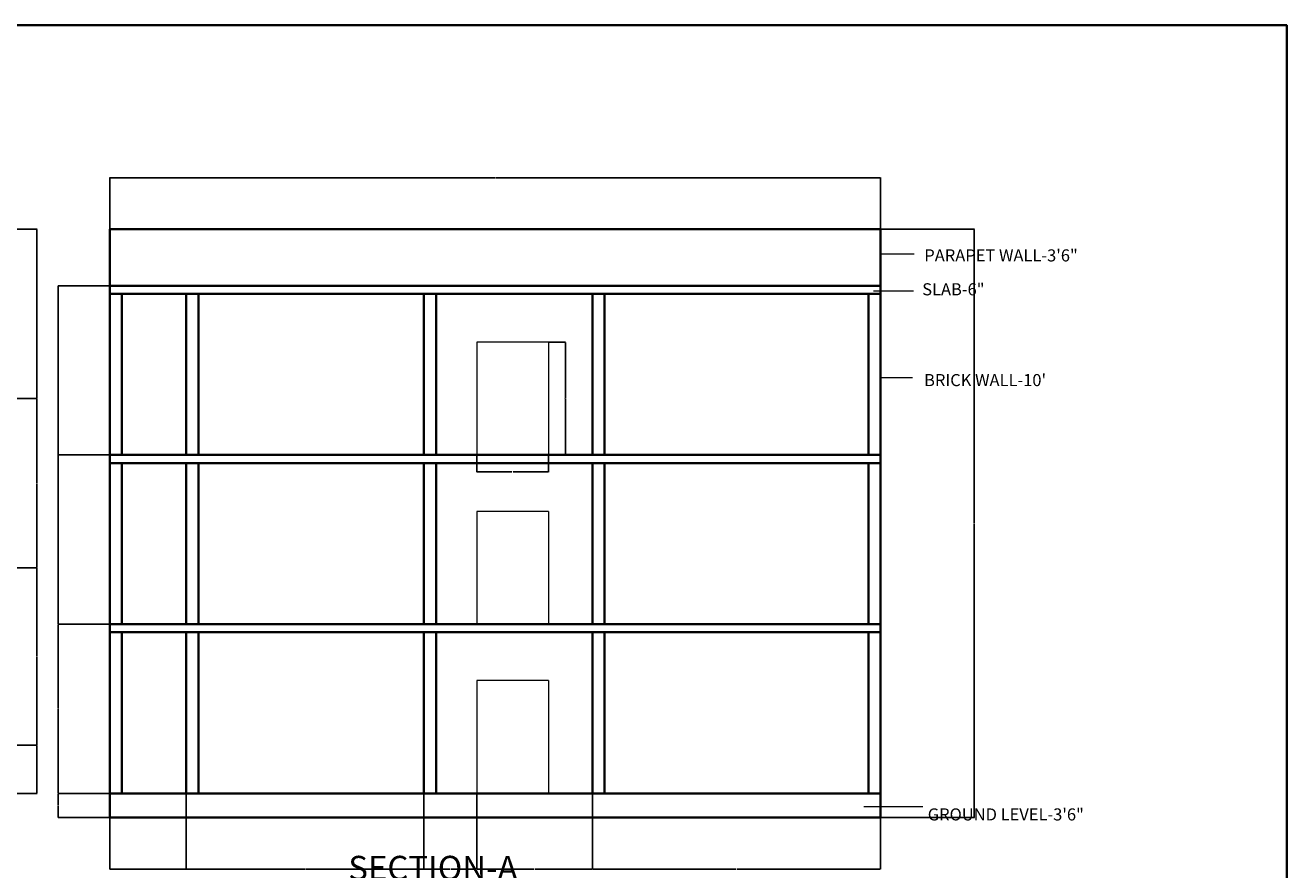
# Model space of a CAD drawing. Units: inches. Extents: x 1824 to 3509, y 619 to 2294.
# Tile 12 of 12: x 2570 to 3509, y 1665 to 2294. Entities that reach past the tile are written whole.
import ezdxf

# ---------------------------------------------------------------- set-up
doc = ezdxf.new("R2010")
doc.units = ezdxf.units.IN
for name, color, linetype, lineweight in [('A-ANNO-DIMS', 2, 'Continuous', 18), ('A-ANNO-SYMB', 7, 'Continuous', 18), ('A-ANNO-TEXT', 7, 'Continuous', 25), ('A-ANNO-TTLB', 7, 'Continuous', 35), ('A-SECT', 7, 'Continuous', 35), ('A-SECT-DOOR', 3, 'Continuous', 18)]:
    doc.layers.add(name, color=color, linetype=linetype, lineweight=lineweight)
doc.styles.get("Standard").update_dxf_attribs({"font": 'arial.ttf'})
doc.dimstyles.get("Standard").update_dxf_attribs({"dimtxt": 0.18, "dimasz": 0.18, "dimexe": 0.18, "dimexo": 0.0625, "dimgap": 0.09, "dimtad": 0, "dimtih": 1, "dimtoh": 1, "dimdec": 4, "dimzin": 0, "dimdsep": 46, "dimtxsty": 'Standard', "dimcen": 0.09, "dimadec": 0, "dimazin": 0, "dimtfac": 1, "dimtdec": 4, "dimtofl": 0, "dimtmove": 0, "dimatfit": 3, "dimfxl": 1, "dimtolj": 1, "dimtzin": 0, "dimarcsym": 0})

# ---------------------------------------------------------------- blocks, each defined once
blk = doc.blocks.new('DOOR-OPENING-SECT')
for p, q in [((0, 84), (0, 0)), ((53.41, 84), (0, 84)), ((53.41, 84), (53.41, 0))]:
    blk.add_line(p, q)
blk = doc.blocks.new('*D48')
at = {"layer": 'A-ANNO-DIMS', "color": 0, "lineweight": -2, "transparency": 16777216}
for p, q in [((2959.55, 2057.75), (2972.27, 2057.75)), ((2972.09, 2057.57), (2972.09, 2015.94)), ((2972.09, 1973.93), (2972.09, 2015.57)), ((2959.55, 1973.75), (2972.27, 1973.75))]:
    blk.add_line(p, q, dxfattribs=at)
at = {"layer": 'A-ANNO-DIMS', "color": 0, "transparency": 16777216}
for points in [[(2972.06, 2057.57), (2972.12, 2057.57), (2972.09, 2057.75)], [(2972.06, 1973.93), (2972.12, 1973.93), (2972.09, 1973.75)]]:
    blk.add_solid(points, dxfattribs=at)
at = {"layer": 'Defpoints', "color": 0, "transparency": 16777216}
for p in [(2959.49, 2057.75), (2972.09, 2057.75), (2959.49, 1973.75)]:
    blk.add_point(p, dxfattribs=at)
at = {"layer": 'A-ANNO-DIMS', "color": 0, "transparency": 16777216, "insert": (2972.09, 2015.75), "char_height": 0.18, "attachment_point": 5}
blk.add_mtext('\\A1;OPENING 84 TYP.', dxfattribs=at)
blk = doc.blocks.new('*D49')
at = {"layer": 'A-ANNO-DIMS', "color": 0, "lineweight": -2, "transparency": 16777216}
for p, q in [((2906.08, 1973.69), (2906.08, 1960.97)), ((2959.49, 1973.69), (2959.49, 1960.97)), ((2906.26, 1961.15), (2932.25, 1961.15)), ((2959.31, 1961.15), (2933.31, 1961.15))]:
    blk.add_line(p, q, dxfattribs=at)
at = {"layer": 'A-ANNO-DIMS', "color": 0, "transparency": 16777216}
for points in [[(2906.26, 1961.18), (2906.26, 1961.12), (2906.08, 1961.15)], [(2959.31, 1961.18), (2959.31, 1961.12), (2959.49, 1961.15)]]:
    blk.add_solid(points, dxfattribs=at)
at = {"layer": 'Defpoints', "color": 0, "transparency": 16777216}
for p in [(2906.08, 1973.75), (2959.49, 1973.75), (2959.49, 1961.15)]:
    blk.add_point(p, dxfattribs=at)
at = {"layer": 'A-ANNO-DIMS', "color": 0, "transparency": 16777216, "insert": (2932.78, 1961.15), "char_height": 0.18, "attachment_point": 5}
blk.add_mtext('\\A1;53 TYP.', dxfattribs=at)
blk = doc.blocks.new('*D126')
at = {"layer": 'A-ANNO-DIMS', "color": 0, "lineweight": -2, "transparency": 16777216}
for p, q in [((2447.72, 1757.75), (2578.67, 1757.75)), ((2578.49, 1757.57), (2578.49, 1739.93)), ((2578.49, 1721.93), (2578.49, 1739.57)), ((2523.15, 1721.75), (2578.67, 1721.75))]:
    blk.add_line(p, q, dxfattribs=at)
at = {"layer": 'A-ANNO-DIMS', "color": 0, "transparency": 16777216}
for points in [[(2578.46, 1757.57), (2578.52, 1757.57), (2578.49, 1757.75)], [(2578.46, 1721.93), (2578.52, 1721.93), (2578.49, 1721.75)]]:
    blk.add_solid(points, dxfattribs=at)
at = {"layer": 'Defpoints', "color": 0, "transparency": 16777216}
for p in [(2447.66, 1757.75), (2578.49, 1757.75), (2523.09, 1721.75)]:
    blk.add_point(p, dxfattribs=at)
at = {"layer": 'A-ANNO-DIMS', "color": 0, "transparency": 16777216, "insert": (2578.49, 1739.75), "char_height": 0.18, "attachment_point": 5}
blk.add_mtext('\\A1;36', dxfattribs=at)
blk = doc.blocks.new('*D127')
at = {"layer": 'A-ANNO-DIMS', "color": 0, "lineweight": -2, "transparency": 16777216}
for p, q in [((2547.15, 1889.75), (2578.67, 1889.75)), ((2578.49, 1889.57), (2578.49, 1823.93)), ((2578.49, 1757.93), (2578.49, 1823.57)), ((2447.72, 1757.75), (2578.67, 1757.75))]:
    blk.add_line(p, q, dxfattribs=at)
at = {"layer": 'A-ANNO-DIMS', "color": 0, "transparency": 16777216}
for points in [[(2578.46, 1889.57), (2578.52, 1889.57), (2578.49, 1889.75)], [(2578.46, 1757.93), (2578.52, 1757.93), (2578.49, 1757.75)]]:
    blk.add_solid(points, dxfattribs=at)
at = {"layer": 'Defpoints', "color": 0, "transparency": 16777216}
for p in [(2547.09, 1889.75), (2578.49, 1889.75), (2447.66, 1757.75)]:
    blk.add_point(p, dxfattribs=at)
at = {"layer": 'A-ANNO-DIMS', "color": 0, "transparency": 16777216, "insert": (2578.49, 1823.75), "char_height": 0.18, "attachment_point": 5}
blk.add_mtext('\\A1;132', dxfattribs=at)
blk = doc.blocks.new('*D128')
at = {"layer": 'A-ANNO-DIMS', "color": 0, "lineweight": -2, "transparency": 16777216}
for p, q in [((2547.15, 2015.75), (2578.67, 2015.75)), ((2578.49, 2015.57), (2578.49, 1952.93)), ((2578.49, 1889.93), (2578.49, 1952.57)), ((2547.15, 1889.75), (2578.67, 1889.75))]:
    blk.add_line(p, q, dxfattribs=at)
at = {"layer": 'A-ANNO-DIMS', "color": 0, "transparency": 16777216}
for points in [[(2578.46, 2015.57), (2578.52, 2015.57), (2578.49, 2015.75)], [(2578.46, 1889.93), (2578.52, 1889.93), (2578.49, 1889.75)]]:
    blk.add_solid(points, dxfattribs=at)
at = {"layer": 'Defpoints', "color": 0, "transparency": 16777216}
for p in [(2547.09, 2015.75), (2578.49, 2015.75), (2547.09, 1889.75)]:
    blk.add_point(p, dxfattribs=at)
at = {"layer": 'A-ANNO-DIMS', "color": 0, "transparency": 16777216, "insert": (2578.49, 1952.75), "char_height": 0.18, "attachment_point": 5}
blk.add_mtext('\\A1;126', dxfattribs=at)
blk = doc.blocks.new('*D129')
at = {"layer": 'A-ANNO-DIMS', "color": 0, "lineweight": -2, "transparency": 16777216}
for p, q in [((2547.15, 2141.75), (2578.67, 2141.75)), ((2578.49, 2141.57), (2578.49, 2078.93)), ((2578.49, 2015.93), (2578.49, 2078.57)), ((2547.15, 2015.75), (2578.67, 2015.75))]:
    blk.add_line(p, q, dxfattribs=at)
at = {"layer": 'A-ANNO-DIMS', "color": 0, "transparency": 16777216}
for points in [[(2578.46, 2141.57), (2578.52, 2141.57), (2578.49, 2141.75)], [(2578.46, 2015.93), (2578.52, 2015.93), (2578.49, 2015.75)]]:
    blk.add_solid(points, dxfattribs=at)
at = {"layer": 'Defpoints', "color": 0, "transparency": 16777216}
for p in [(2547.09, 2141.75), (2578.49, 2141.75), (2547.09, 2015.75)]:
    blk.add_point(p, dxfattribs=at)
at = {"layer": 'A-ANNO-DIMS', "color": 0, "transparency": 16777216, "insert": (2578.49, 2078.75), "char_height": 0.18, "attachment_point": 5}
blk.add_mtext('\\A1;126', dxfattribs=at)
blk = doc.blocks.new('*D130')
at = {"layer": 'A-ANNO-DIMS', "color": 0, "lineweight": -2, "transparency": 16777216}
for p, q in [((2632.73, 2141.81), (2632.73, 2180.23)), ((2632.91, 2180.05), (2919.44, 2180.05)), ((3206.55, 2180.05), (2920.02, 2180.05)), ((3206.73, 2141.81), (3206.73, 2180.23))]:
    blk.add_line(p, q, dxfattribs=at)
at = {"layer": 'A-ANNO-DIMS', "color": 0, "transparency": 16777216}
for points in [[(2632.91, 2180.08), (2632.91, 2180.02), (2632.73, 2180.05)], [(3206.55, 2180.08), (3206.55, 2180.02), (3206.73, 2180.05)]]:
    blk.add_solid(points, dxfattribs=at)
at = {"layer": 'Defpoints', "color": 0, "transparency": 16777216}
for p in [(3206.73, 2180.05), (2632.73, 2141.75), (3206.73, 2141.75)]:
    blk.add_point(p, dxfattribs=at)
at = {"layer": 'A-ANNO-DIMS', "color": 0, "transparency": 16777216, "insert": (2919.73, 2180.05), "char_height": 0.18, "attachment_point": 5}
blk.add_mtext('\\A1;574', dxfattribs=at)
blk = doc.blocks.new('*D131')
at = {"layer": 'A-ANNO-DIMS', "color": 0, "lineweight": -2, "transparency": 16777216}
for p, q in [((3206.79, 2141.75), (3276.71, 2141.75)), ((3276.53, 2141.57), (3276.53, 1922.93)), ((3276.53, 1703.93), (3276.53, 1922.57)), ((3206.79, 1703.75), (3276.71, 1703.75))]:
    blk.add_line(p, q, dxfattribs=at)
at = {"layer": 'A-ANNO-DIMS', "color": 0, "transparency": 16777216}
for points in [[(3276.5, 2141.57), (3276.56, 2141.57), (3276.53, 2141.75)], [(3276.5, 1703.93), (3276.56, 1703.93), (3276.53, 1703.75)]]:
    blk.add_solid(points, dxfattribs=at)
at = {"layer": 'Defpoints', "color": 0, "transparency": 16777216}
for p in [(3206.73, 2141.75), (3276.53, 2141.75), (3206.73, 1703.75)]:
    blk.add_point(p, dxfattribs=at)
at = {"layer": 'A-ANNO-DIMS', "color": 0, "transparency": 16777216, "insert": (3276.53, 1922.75), "char_height": 0.18, "attachment_point": 5}
blk.add_mtext('\\A1;438', dxfattribs=at)
blk = doc.blocks.new('*D132')
at = {"layer": 'A-ANNO-DIMS', "color": 0, "lineweight": -2, "transparency": 16777216}
for p, q in [((2632.67, 1721.75), (2594.25, 1721.75)), ((2594.43, 1721.57), (2594.43, 1712.93)), ((2594.43, 1703.93), (2594.43, 1712.57)), ((2632.67, 1703.75), (2594.25, 1703.75))]:
    blk.add_line(p, q, dxfattribs=at)
at = {"layer": 'A-ANNO-DIMS', "color": 0, "transparency": 16777216}
for points in [[(2594.4, 1721.57), (2594.46, 1721.57), (2594.43, 1721.75)], [(2594.4, 1703.93), (2594.46, 1703.93), (2594.43, 1703.75)]]:
    blk.add_solid(points, dxfattribs=at)
at = {"layer": 'Defpoints', "color": 0, "transparency": 16777216}
for p in [(2594.43, 1721.75), (2632.73, 1721.75), (2632.73, 1703.75)]:
    blk.add_point(p, dxfattribs=at)
at = {"layer": 'A-ANNO-DIMS', "color": 0, "transparency": 16777216, "insert": (2594.43, 1712.75), "char_height": 0.18, "attachment_point": 5}
blk.add_mtext('\\A1;18', dxfattribs=at)
blk = doc.blocks.new('*D133')
at = {"layer": 'A-ANNO-DIMS', "color": 0, "lineweight": -2, "transparency": 16777216}
for p, q in [((2632.67, 1847.75), (2594.25, 1847.75)), ((2594.43, 1847.57), (2594.43, 1784.93)), ((2594.43, 1721.93), (2594.43, 1784.57)), ((2632.67, 1721.75), (2594.25, 1721.75))]:
    blk.add_line(p, q, dxfattribs=at)
at = {"layer": 'A-ANNO-DIMS', "color": 0, "transparency": 16777216}
for points in [[(2594.4, 1847.57), (2594.46, 1847.57), (2594.43, 1847.75)], [(2594.4, 1721.93), (2594.46, 1721.93), (2594.43, 1721.75)]]:
    blk.add_solid(points, dxfattribs=at)
at = {"layer": 'Defpoints', "color": 0, "transparency": 16777216}
for p in [(2594.43, 1847.75), (2632.73, 1847.75), (2632.73, 1721.75)]:
    blk.add_point(p, dxfattribs=at)
at = {"layer": 'A-ANNO-DIMS', "color": 0, "transparency": 16777216, "insert": (2594.43, 1784.75), "char_height": 0.18, "attachment_point": 5}
blk.add_mtext('\\A1;126', dxfattribs=at)
blk = doc.blocks.new('*D134')
at = {"layer": 'A-ANNO-DIMS', "color": 0, "lineweight": -2, "transparency": 16777216}
for p, q in [((2632.67, 1973.75), (2594.25, 1973.75)), ((2594.43, 1973.57), (2594.43, 1910.93)), ((2594.43, 1847.93), (2594.43, 1910.57)), ((2632.67, 1847.75), (2594.25, 1847.75))]:
    blk.add_line(p, q, dxfattribs=at)
at = {"layer": 'A-ANNO-DIMS', "color": 0, "transparency": 16777216}
for points in [[(2594.4, 1973.57), (2594.46, 1973.57), (2594.43, 1973.75)], [(2594.4, 1847.93), (2594.46, 1847.93), (2594.43, 1847.75)]]:
    blk.add_solid(points, dxfattribs=at)
at = {"layer": 'Defpoints', "color": 0, "transparency": 16777216}
for p in [(2594.43, 1973.75), (2632.73, 1973.75), (2632.73, 1847.75)]:
    blk.add_point(p, dxfattribs=at)
at = {"layer": 'A-ANNO-DIMS', "color": 0, "transparency": 16777216, "insert": (2594.43, 1910.75), "char_height": 0.18, "attachment_point": 5}
blk.add_mtext('\\A1;126', dxfattribs=at)
blk = doc.blocks.new('*D135')
at = {"layer": 'A-ANNO-DIMS', "color": 0, "lineweight": -2, "transparency": 16777216}
for p, q in [((2632.67, 2099.75), (2594.25, 2099.75)), ((2594.43, 2099.57), (2594.43, 2036.93)), ((2594.43, 1973.93), (2594.43, 2036.57)), ((2632.67, 1973.75), (2594.25, 1973.75))]:
    blk.add_line(p, q, dxfattribs=at)
at = {"layer": 'A-ANNO-DIMS', "color": 0, "transparency": 16777216}
for points in [[(2594.4, 2099.57), (2594.46, 2099.57), (2594.43, 2099.75)], [(2594.4, 1973.93), (2594.46, 1973.93), (2594.43, 1973.75)]]:
    blk.add_solid(points, dxfattribs=at)
at = {"layer": 'Defpoints', "color": 0, "transparency": 16777216}
for p in [(2594.43, 2099.75), (2632.73, 2099.75), (2632.73, 1973.75)]:
    blk.add_point(p, dxfattribs=at)
at = {"layer": 'A-ANNO-DIMS', "color": 0, "transparency": 16777216, "insert": (2594.43, 2036.75), "char_height": 0.18, "attachment_point": 5}
blk.add_mtext('\\A1;126', dxfattribs=at)
blk = doc.blocks.new('*D136')
at = {"layer": 'A-ANNO-DIMS', "color": 0, "lineweight": -2, "transparency": 16777216}
for p, q in [((2689.73, 1721.69), (2689.73, 1665.27)), ((2632.73, 1703.69), (2632.73, 1665.27)), ((2632.91, 1665.45), (2661.01, 1665.45)), ((2689.55, 1665.45), (2661.45, 1665.45))]:
    blk.add_line(p, q, dxfattribs=at)
at = {"layer": 'A-ANNO-DIMS', "color": 0, "transparency": 16777216}
for points in [[(2632.91, 1665.48), (2632.91, 1665.42), (2632.73, 1665.45)], [(2689.55, 1665.48), (2689.55, 1665.42), (2689.73, 1665.45)]]:
    blk.add_solid(points, dxfattribs=at)
at = {"layer": 'Defpoints', "color": 0, "transparency": 16777216}
for p in [(2689.73, 1721.75), (2632.73, 1703.75), (2689.73, 1665.45)]:
    blk.add_point(p, dxfattribs=at)
at = {"layer": 'A-ANNO-DIMS', "color": 0, "transparency": 16777216, "insert": (2661.23, 1665.45), "char_height": 0.18, "attachment_point": 5}
blk.add_mtext('\\A1;57', dxfattribs=at)
blk = doc.blocks.new('*D137')
at = {"layer": 'A-ANNO-DIMS', "color": 0, "lineweight": -2, "transparency": 16777216}
for p, q in [((2689.73, 1721.69), (2689.73, 1665.27)), ((2866.73, 1721.69), (2866.73, 1665.27)), ((2689.91, 1665.45), (2777.95, 1665.45)), ((2866.55, 1665.45), (2778.51, 1665.45))]:
    blk.add_line(p, q, dxfattribs=at)
at = {"layer": 'A-ANNO-DIMS', "color": 0, "transparency": 16777216}
for points in [[(2689.91, 1665.48), (2689.91, 1665.42), (2689.73, 1665.45)], [(2866.55, 1665.48), (2866.55, 1665.42), (2866.73, 1665.45)]]:
    blk.add_solid(points, dxfattribs=at)
at = {"layer": 'Defpoints', "color": 0, "transparency": 16777216}
for p in [(2689.73, 1721.75), (2866.73, 1721.75), (2866.73, 1665.45)]:
    blk.add_point(p, dxfattribs=at)
at = {"layer": 'A-ANNO-DIMS', "color": 0, "transparency": 16777216, "insert": (2778.23, 1665.45), "char_height": 0.18, "attachment_point": 5}
blk.add_mtext('\\A1;177', dxfattribs=at)
blk = doc.blocks.new('*D138')
at = {"layer": 'A-ANNO-DIMS', "color": 0, "lineweight": -2, "transparency": 16777216}
for p, q in [((2866.73, 1721.69), (2866.73, 1665.27)), ((2906.08, 1721.69), (2906.08, 1665.27)), ((2866.91, 1665.45), (2886.01, 1665.45)), ((2905.9, 1665.45), (2886.8, 1665.45))]:
    blk.add_line(p, q, dxfattribs=at)
at = {"layer": 'A-ANNO-DIMS', "color": 0, "transparency": 16777216}
for points in [[(2866.91, 1665.48), (2866.91, 1665.42), (2866.73, 1665.45)], [(2905.9, 1665.48), (2905.9, 1665.42), (2906.08, 1665.45)]]:
    blk.add_solid(points, dxfattribs=at)
at = {"layer": 'Defpoints', "color": 0, "transparency": 16777216}
for p in [(2866.73, 1721.75), (2906.08, 1721.75), (2906.08, 1665.45)]:
    blk.add_point(p, dxfattribs=at)
at = {"layer": 'A-ANNO-DIMS', "color": 0, "transparency": 16777216, "insert": (2886.4, 1665.45), "char_height": 0.18, "attachment_point": 5}
blk.add_mtext('\\A1;39.35', dxfattribs=at)
blk = doc.blocks.new('*D139')
at = {"layer": 'A-ANNO-DIMS', "color": 0, "lineweight": -2, "transparency": 16777216}
for p, q in [((2906.08, 1721.69), (2906.08, 1665.27)), ((2992.23, 1721.69), (2992.23, 1665.27)), ((2906.26, 1665.45), (2948.76, 1665.45)), ((2992.05, 1665.45), (2949.55, 1665.45))]:
    blk.add_line(p, q, dxfattribs=at)
at = {"layer": 'A-ANNO-DIMS', "color": 0, "transparency": 16777216}
for points in [[(2906.26, 1665.48), (2906.26, 1665.42), (2906.08, 1665.45)], [(2992.05, 1665.48), (2992.05, 1665.42), (2992.23, 1665.45)]]:
    blk.add_solid(points, dxfattribs=at)
at = {"layer": 'Defpoints', "color": 0, "transparency": 16777216}
for p in [(2906.08, 1721.75), (2992.23, 1721.75), (2992.23, 1665.45)]:
    blk.add_point(p, dxfattribs=at)
at = {"layer": 'A-ANNO-DIMS', "color": 0, "transparency": 16777216, "insert": (2949.15, 1665.45), "char_height": 0.18, "attachment_point": 5}
blk.add_mtext('\\A1;86.15', dxfattribs=at)
blk = doc.blocks.new('*D140')
at = {"layer": 'A-ANNO-DIMS', "color": 0, "lineweight": -2, "transparency": 16777216}
for p, q in [((2992.23, 1721.69), (2992.23, 1665.27)), ((3206.73, 1703.69), (3206.73, 1665.27)), ((2992.41, 1665.45), (3099.08, 1665.45)), ((3206.55, 1665.45), (3099.87, 1665.45))]:
    blk.add_line(p, q, dxfattribs=at)
at = {"layer": 'A-ANNO-DIMS', "color": 0, "transparency": 16777216}
for points in [[(2992.41, 1665.48), (2992.41, 1665.42), (2992.23, 1665.45)], [(3206.55, 1665.48), (3206.55, 1665.42), (3206.73, 1665.45)]]:
    blk.add_solid(points, dxfattribs=at)
at = {"layer": 'Defpoints', "color": 0, "transparency": 16777216}
for p in [(2992.23, 1721.75), (3206.73, 1703.75), (3206.73, 1665.45)]:
    blk.add_point(p, dxfattribs=at)
at = {"layer": 'A-ANNO-DIMS', "color": 0, "transparency": 16777216, "insert": (3099.48, 1665.45), "char_height": 0.18, "attachment_point": 5}
blk.add_mtext('\\A1;214.5', dxfattribs=at)

msp = doc.modelspace()

# ---------------------------------------------------------------- linework, layer by layer
at = {"layer": 'A-ANNO-SYMB'}
for p, q in [((3206.7282, 2123.5094), (3231.9029, 2123.5094)), ((3201.6012, 2096.0059), (3231.4406, 2096.0059)), ((3206.7282, 2031.315), (3230.6619, 2031.315)), ((3194.4511, 1711.9835), (3238.2318, 1711.9835))]:
    msp.add_line(p, q, dxfattribs=at)
at = {"layer": 'A-ANNO-TTLB'}
msp.add_lwpolyline([(1824.0608, 2293.6614), (3509.3484, 2293.6614), (3509.3484, 619.4665), (1824.0608, 619.4665)], close=True, dxfattribs=at)
at = {"layer": 'A-SECT'}
for p, q in [((2632.7282, 2141.7521), (2632.7282, 1955.7521)), ((3206.7282, 2141.7521), (2632.7282, 2141.7521)), ((3206.7282, 2141.7521), (3206.7282, 1955.7521)), ((3206.7282, 2099.7521), (2632.7282, 2099.7521)), ((3206.7282, 2093.7521), (2632.7282, 2093.7521)), ((2641.7282, 2093.7521), (2641.7282, 1973.7521)), ((2689.7282, 2093.7521), (2689.7282, 1973.7521)), ((2689.7282, 2093.7521), (2689.7282, 1973.7521)), ((2698.7282, 2093.7521), (2698.7282, 1973.7521)), ((2698.7282, 2093.7521), (2698.7282, 1973.7521)), ((2866.7282, 2093.7521), (2866.7282, 1973.7521)), ((2875.7282, 2093.7521), (2875.7282, 1973.7521)), ((2992.2282, 2093.7521), (2992.2282, 1973.7521)), ((3001.2282, 2093.7521), (3001.2282, 1973.7521)), ((3197.7282, 2093.7521), (3197.7282, 1973.7521)), ((2632.7282, 2015.7521), (2632.7282, 1829.7521)), ((2632.7282, 2015.7521), (2632.7282, 1829.7521)), ((3206.7282, 2015.7521), (3206.7282, 1829.7521)), ((3206.7282, 2015.7521), (3206.7282, 1829.7521)), ((3206.7282, 1973.7521), (2632.7282, 1973.7521)), ((3206.7282, 1973.7521), (2632.7282, 1973.7521)), ((3206.7282, 1967.7521), (2632.7282, 1967.7521)), ((3206.7282, 1967.7521), (2632.7282, 1967.7521)), ((2641.7282, 1967.7521), (2641.7282, 1847.7521)), ((2641.7282, 1967.7521), (2641.7282, 1847.7521)), ((2689.7282, 1967.7521), (2689.7282, 1847.7521)), ((2689.7282, 1967.7521), (2689.7282, 1847.7521)), ((2689.7282, 1967.7521), (2689.7282, 1847.7521)), ((2689.7282, 1967.7521), (2689.7282, 1847.7521)), ((2698.7282, 1967.7521), (2698.7282, 1847.7521)), ((2698.7282, 1967.7521), (2698.7282, 1847.7521)), ((2698.7282, 1967.7521), (2698.7282, 1847.7521)), ((2698.7282, 1967.7521), (2698.7282, 1847.7521)), ((2866.7282, 1967.7521), (2866.7282, 1847.7521)), ((2866.7282, 1967.7521), (2866.7282, 1847.7521)), ((2875.7282, 1967.7521), (2875.7282, 1847.7521)), ((2875.7282, 1967.7521), (2875.7282, 1847.7521)), ((2992.2282, 1967.7521), (2992.2282, 1847.7521)), ((2992.2282, 1967.7521), (2992.2282, 1847.7521)), ((3001.2282, 1967.7521), (3001.2282, 1847.7521)), ((3001.2282, 1967.7521), (3001.2282, 1847.7521)), ((3197.7282, 1967.7521), (3197.7282, 1847.7521)), ((3197.7282, 1967.7521), (3197.7282, 1847.7521)), ((2632.7282, 1889.7521), (2632.7282, 1703.7521)), ((3206.7282, 1889.7521), (3206.7282, 1703.7521)), ((3206.7282, 1847.7521), (2632.7282, 1847.7521)), ((3206.7282, 1841.7521), (2632.7282, 1841.7521)), ((2641.7282, 1841.7521), (2641.7282, 1721.7521)), ((2689.7282, 1841.7521), (2689.7282, 1721.7521)), ((2689.7282, 1841.7521), (2689.7282, 1721.7521)), ((2698.7282, 1841.7521), (2698.7282, 1721.7521)), ((2698.7282, 1841.7521), (2698.7282, 1721.7521)), ((2866.7282, 1841.7521), (2866.7282, 1721.7521)), ((2875.7282, 1841.7521), (2875.7282, 1721.7521)), ((2992.2282, 1841.7521), (2992.2282, 1721.7521)), ((3001.2282, 1841.7521), (3001.2282, 1721.7521)), ((3197.7282, 1841.7521), (3197.7282, 1721.7521)), ((3206.7282, 1721.7521), (2632.7282, 1721.7521)), ((3206.7282, 1703.7521), (2632.7282, 1703.7521)), ((3206.7282, 1703.7521), (2632.7282, 1703.7521))]:
    msp.add_line(p, q, dxfattribs=at)

# ---------------------------------------------------------------- block references
at = {"layer": 'A-SECT-DOOR'}
for p in [(2906.078, 1973.752), (2906.078, 1847.752), (2906.078, 1847.752), (2906.078, 1721.752)]:
    msp.add_blockref('DOOR-OPENING-SECT', p, dxfattribs=at)

# ---------------------------------------------------------------- texts
at = {"layer": 'A-ANNO-TEXT', "attachment_point": 1}
for s, width, insert, char_height in [('PARAPET WALL-3\'6"', 341.336967, (3239.4028, 2126.8143), 9), ('SLAB-6"', 59.420797, (3237.8359, 2101.5868), 9), ("BRICK WALL-10'", 146.360884, (3239.2259, 2033.9854), 9), ('GROUND LEVEL-3\'6"', 171.746045, (3241.9663, 1710.647), 9), ('SECTION-A', 244.115567, (2810.3821, 1675.3119), 18)]:
    msp.add_mtext_dynamic_manual_height_columns(s, width=width, gutter_width=12.5, heights=[0], dxfattribs=dict(at, insert=insert, char_height=char_height))

# ---------------------------------------------------------------- dimensions: what is measured, and where the dimension line sits
at = {"layer": 'A-ANNO-DIMS'}
for base, p1, p2, override, picture, middle in [((3206.7282, 2180.0521), (2632.7282, 2141.7521), (3206.7282, 2141.7521), {"dimdec": 0, "dimlfac": 1, "dimrnd": 0, "dimzin": 0, "dimdsep": 46, "dimlunit": 2}, '*D130', (2919.7282, 2180.0521)), ((2689.7282, 1665.4521), (2632.7282, 1703.7521), (2689.7282, 1721.7521), {"dimdec": 0, "dimlfac": 1, "dimrnd": 0, "dimzin": 0, "dimdsep": 46, "dimlunit": 2}, '*D136', (2661.2282, 1665.4521)), ((2866.7282, 1665.4521), (2689.7282, 1721.7521), (2866.7282, 1721.7521), {"dimdec": 0, "dimlfac": 1, "dimrnd": 0, "dimzin": 0, "dimdsep": 46, "dimlunit": 2}, '*D137', (2778.2282, 1665.4521)), ((2906.0784, 1665.4521), (2866.7282, 1721.7521), (2906.0784, 1721.7521), {"dimdec": 2, "dimlfac": 1, "dimrnd": 0, "dimzin": 0, "dimdsep": 46, "dimlunit": 2}, '*D138', (2886.4033, 1665.4521)), ((2992.2282, 1665.4521), (2906.0784, 1721.7521), (2992.2282, 1721.7521), {"dimdec": 2, "dimlfac": 1, "dimrnd": 0, "dimzin": 0, "dimdsep": 46, "dimlunit": 2}, '*D139', (2949.1533, 1665.4521)), ((3206.7282, 1665.4521), (2992.2282, 1721.7521), (3206.7282, 1703.7521), {"dimdec": 1, "dimlfac": 1, "dimrnd": 0, "dimzin": 0, "dimdsep": 46, "dimlunit": 2}, '*D140', (3099.4782, 1665.4521))]:
    dim = msp.add_linear_dim(base=base, p1=p1, p2=p2, dimstyle='Standard', override=override, dxfattribs=at)
    dim.commit()
    dim.dimension.update_dxf_attribs({"geometry": picture, "text_midpoint": middle})
for base, p1, p2, picture, middle in [((2578.4899, 2141.7521), (2547.0899, 2015.7521), (2547.0899, 2141.7521), '*D129', (2578.4899, 2078.7521)), ((3276.5318, 2141.7521), (3206.7282, 1703.7521), (3206.7282, 2141.7521), '*D131', (3276.5318, 1922.7521)), ((2594.4282, 2099.7521), (2632.7282, 1973.7521), (2632.7282, 2099.7521), '*D135', (2594.4282, 2036.7521)), ((2578.4899, 2015.7521), (2547.0899, 1889.7521), (2547.0899, 2015.7521), '*D128', (2578.4899, 1952.7521)), ((2594.4282, 1973.7521), (2632.7282, 1847.7521), (2632.7282, 1973.7521), '*D134', (2594.4282, 1910.7521)), ((2578.4899, 1889.7521), (2447.6578, 1757.7521), (2547.0899, 1889.7521), '*D127', (2578.4899, 1823.7521)), ((2594.4282, 1847.7521), (2632.7282, 1721.7521), (2632.7282, 1847.7521), '*D133', (2594.4282, 1784.7521)), ((2578.4899, 1757.7521), (2523.0899, 1721.7521), (2447.6578, 1757.7521), '*D126', (2578.4899, 1739.7521)), ((2594.4282, 1721.7521), (2632.7282, 1703.7521), (2632.7282, 1721.7521), '*D132', (2594.4282, 1712.7521))]:
    dim = msp.add_linear_dim(base=base, p1=p1, p2=p2, angle=90, dimstyle='Standard', override={"dimdec": 0, "dimlfac": 1, "dimrnd": 0, "dimzin": 0, "dimdsep": 46, "dimlunit": 2}, dxfattribs=at)
    dim.commit()
    dim.dimension.update_dxf_attribs({"geometry": picture, "text_midpoint": middle})
dim = msp.add_linear_dim(base=(2972.0861, 2057.7521), p1=(2959.4861, 1973.7521), p2=(2959.4861, 2057.7521), angle=90, text='OPENING <> TYP.', dimstyle='Standard', override={"dimdec": 0, "dimlfac": 1, "dimrnd": 0, "dimzin": 0, "dimdsep": 46, "dimlunit": 2}, dxfattribs=at)
dim.commit()
dim.dimension.update_dxf_attribs({"geometry": '*D48', "text_midpoint": (2972.0861, 2015.7521)})
dim = msp.add_linear_dim(base=(2959.4861, 1961.1521), p1=(2906.0784, 1973.7521), p2=(2959.4861, 1973.7521), text='<> TYP.', dimstyle='Standard', override={"dimdec": 0, "dimlfac": 1, "dimrnd": 0, "dimzin": 0, "dimdsep": 46, "dimlunit": 2}, dxfattribs=at)
dim.commit()
dim.dimension.update_dxf_attribs({"geometry": '*D49', "text_midpoint": (2932.7822, 1961.1521)})

doc.saveas('drawing.dxf')
